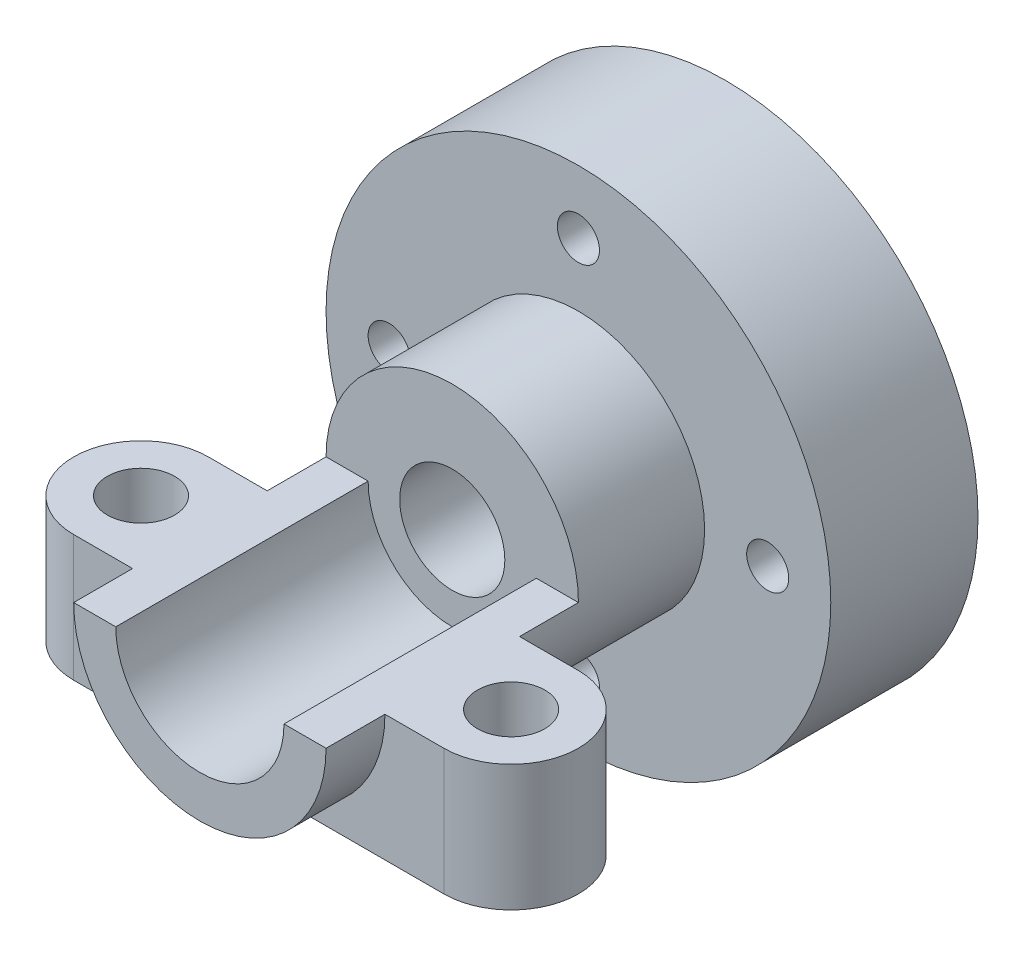
ISO-10303-21;
HEADER;
FILE_DESCRIPTION(('STEP AP214'),'2;1');
FILE_NAME('part.step','',(''),(''),'','','');
FILE_SCHEMA(('AUTOMOTIVE_DESIGN { 1 0 10303 214 1 1 1 1 }'));
ENDSEC;
DATA;
#1=APPLICATION_CONTEXT('core data for automotive mechanical design processes');
#2=APPLICATION_PROTOCOL_DEFINITION('international standard','automotive_design',2000,#1);
#3=PRODUCT_CONTEXT('',#1,'mechanical');
#4=PRODUCT('Part','Part','',(#3));
#5=PRODUCT_RELATED_PRODUCT_CATEGORY('part','',(#4));
#6=PRODUCT_DEFINITION_FORMATION('','',#4);
#7=PRODUCT_DEFINITION_CONTEXT('part definition',#1,'design');
#8=PRODUCT_DEFINITION('design','',#6,#7);
#9=PRODUCT_DEFINITION_SHAPE('','',#8);
#10=(LENGTH_UNIT() NAMED_UNIT(*) SI_UNIT(.MILLI.,.METRE.));
#11=(NAMED_UNIT(*) PLANE_ANGLE_UNIT() SI_UNIT($,.RADIAN.));
#12=(NAMED_UNIT(*) SI_UNIT($,.STERADIAN.) SOLID_ANGLE_UNIT());
#13=UNCERTAINTY_MEASURE_WITH_UNIT(LENGTH_MEASURE(1.E-05),#10,'distance_accuracy_value','');
#14=(GEOMETRIC_REPRESENTATION_CONTEXT(3) GLOBAL_UNCERTAINTY_ASSIGNED_CONTEXT((#13)) GLOBAL_UNIT_ASSIGNED_CONTEXT((#10,
#11,#12)) REPRESENTATION_CONTEXT('',''));
#15=CARTESIAN_POINT('',(0.,0.,0.));
#16=DIRECTION('',(0.,0.,1.));
#17=DIRECTION('',(1.,0.,0.));
#18=AXIS2_PLACEMENT_3D('',#15,#16,#17);
#19=CARTESIAN_POINT('',(-30.,0.,90.));
#20=DIRECTION('',(0.,-1.,0.));
#21=DIRECTION('',(0.,0.,-1.));
#22=AXIS2_PLACEMENT_3D('',#19,#20,#21);
#23=PLANE('',#22);
#24=CARTESIAN_POINT('',(44.,0.,60.));
#25=DIRECTION('',(0.,1.,0.));
#26=DIRECTION('',(0.,0.,1.));
#27=AXIS2_PLACEMENT_3D('',#24,#25,#26);
#28=CIRCLE('',#27,8.);
#29=CARTESIAN_POINT('',(44.,0.,68.));
#30=VERTEX_POINT('',#29);
#31=EDGE_CURVE('E163',#30,#30,#28,.T.);
#32=ORIENTED_EDGE('',*,*,#31,.F.);
#33=EDGE_LOOP('',(#32));
#34=FACE_BOUND('',#33,.T.);
#35=DIRECTION('',(0.,0.,1.));
#36=VECTOR('',#35,1.);
#37=CARTESIAN_POINT('',(20.,0.,30.));
#38=LINE('',#37,#36);
#39=CARTESIAN_POINT('',(20.,0.,30.));
#40=VERTEX_POINT('',#39);
#41=CARTESIAN_POINT('',(20.,0.,90.));
#42=VERTEX_POINT('',#41);
#43=EDGE_CURVE('E198',#40,#42,#38,.T.);
#44=ORIENTED_EDGE('',*,*,#43,.T.);
#45=DIRECTION('',(-1.,0.,0.));
#46=VECTOR('',#45,1.);
#47=CARTESIAN_POINT('',(-30.,0.,90.));
#48=LINE('',#47,#46);
#49=CARTESIAN_POINT('',(30.,0.,90.));
#50=VERTEX_POINT('',#49);
#51=EDGE_CURVE('E230',#50,#42,#48,.T.);
#52=ORIENTED_EDGE('',*,*,#51,.F.);
#53=DIRECTION('',(0.,0.,-1.));
#54=VECTOR('',#53,1.);
#55=CARTESIAN_POINT('',(30.,0.,90.));
#56=LINE('',#55,#54);
#57=CARTESIAN_POINT('',(30.,0.,76.));
#58=VERTEX_POINT('',#57);
#59=EDGE_CURVE('E238',#50,#58,#56,.T.);
#60=ORIENTED_EDGE('',*,*,#59,.T.);
#61=DIRECTION('',(1.,0.,0.));
#62=VECTOR('',#61,1.);
#63=CARTESIAN_POINT('',(30.,0.,76.));
#64=LINE('',#63,#62);
#65=CARTESIAN_POINT('',(44.,0.,76.));
#66=VERTEX_POINT('',#65);
#67=EDGE_CURVE('E151',#58,#66,#64,.T.);
#68=ORIENTED_EDGE('',*,*,#67,.T.);
#69=CARTESIAN_POINT('',(44.,0.,60.));
#70=DIRECTION('',(0.,1.,0.));
#71=DIRECTION('',(0.,0.,1.));
#72=AXIS2_PLACEMENT_3D('',#69,#70,#71);
#73=CIRCLE('',#72,16.);
#74=CARTESIAN_POINT('',(44.,0.,44.));
#75=VERTEX_POINT('',#74);
#76=EDGE_CURVE('E161',#66,#75,#73,.T.);
#77=ORIENTED_EDGE('',*,*,#76,.T.);
#78=DIRECTION('',(-1.,0.,0.));
#79=VECTOR('',#78,1.);
#80=CARTESIAN_POINT('',(44.,0.,44.));
#81=LINE('',#80,#79);
#82=CARTESIAN_POINT('',(30.,0.,44.));
#83=VERTEX_POINT('',#82);
#84=EDGE_CURVE('E146',#75,#83,#81,.T.);
#85=ORIENTED_EDGE('',*,*,#84,.T.);
#86=CARTESIAN_POINT('',(30.,0.,30.));
#87=VERTEX_POINT('',#86);
#88=EDGE_CURVE('E240',#83,#87,#56,.T.);
#89=ORIENTED_EDGE('',*,*,#88,.T.);
#90=DIRECTION('',(-1.,0.,0.));
#91=VECTOR('',#90,1.);
#92=CARTESIAN_POINT('',(-30.,0.,30.));
#93=LINE('',#92,#91);
#94=EDGE_CURVE('E226',#87,#40,#93,.T.);
#95=ORIENTED_EDGE('',*,*,#94,.T.);
#96=EDGE_LOOP('',(#44,#52,#60,#68,#77,#85,#89,#95));
#97=FACE_BOUND('',#96,.T.);
#98=ADVANCED_FACE('F44',(#34,#97),#23,.F.);
#99=CARTESIAN_POINT('',(0.,0.,30.));
#100=DIRECTION('',(0.,0.,-1.));
#101=DIRECTION('',(-1.,0.,0.));
#102=AXIS2_PLACEMENT_3D('',#99,#100,#101);
#103=CYLINDRICAL_SURFACE('',#102,30.);
#104=DIRECTION('',(0.,0.,-1.));
#105=VECTOR('',#104,1.);
#106=CARTESIAN_POINT('',(-30.,0.,90.));
#107=LINE('',#106,#105);
#108=CARTESIAN_POINT('',(-30.,0.,90.));
#109=VERTEX_POINT('',#108);
#110=CARTESIAN_POINT('',(-30.,0.,76.));
#111=VERTEX_POINT('',#110);
#112=EDGE_CURVE('E232',#109,#111,#107,.T.);
#113=ORIENTED_EDGE('',*,*,#112,.T.);
#114=CARTESIAN_POINT('',(0.,0.,76.));
#115=DIRECTION('',(0.,0.,1.));
#116=DIRECTION('',(1.,0.,0.));
#117=AXIS2_PLACEMENT_3D('',#114,#115,#116);
#118=CIRCLE('',#117,30.);
#119=CARTESIAN_POINT('',(0.,-30.,76.));
#120=VERTEX_POINT('',#119);
#121=EDGE_CURVE('E66',#111,#120,#118,.T.);
#122=ORIENTED_EDGE('',*,*,#121,.T.);
#123=EDGE_CURVE('E184',#120,#58,#118,.T.);
#124=ORIENTED_EDGE('',*,*,#123,.T.);
#125=ORIENTED_EDGE('',*,*,#59,.F.);
#126=CARTESIAN_POINT('',(0.,0.,90.));
#127=DIRECTION('',(0.,0.,1.));
#128=DIRECTION('',(1.,0.,0.));
#129=AXIS2_PLACEMENT_3D('',#126,#127,#128);
#130=CIRCLE('',#129,30.);
#131=EDGE_CURVE('E221',#109,#50,#130,.T.);
#132=ORIENTED_EDGE('',*,*,#131,.F.);
#133=EDGE_LOOP('',(#113,#122,#124,#125,#132));
#134=FACE_BOUND('',#133,.T.);
#135=ADVANCED_FACE('F273',(#134),#103,.T.);
#136=CARTESIAN_POINT('',(0.,0.,-35.));
#137=DIRECTION('',(0.,0.,1.));
#138=DIRECTION('',(1.,0.,0.));
#139=AXIS2_PLACEMENT_3D('',#136,#137,#138);
#140=CYLINDRICAL_SURFACE('',#139,60.);
#141=CARTESIAN_POINT('',(0.,0.,-35.));
#142=DIRECTION('',(0.,0.,1.));
#143=DIRECTION('',(1.,0.,0.));
#144=AXIS2_PLACEMENT_3D('',#141,#142,#143);
#145=CIRCLE('',#144,60.);
#146=CARTESIAN_POINT('',(60.,0.,-35.));
#147=VERTEX_POINT('',#146);
#148=EDGE_CURVE('E53',#147,#147,#145,.T.);
#149=ORIENTED_EDGE('',*,*,#148,.T.);
#150=EDGE_LOOP('',(#149));
#151=FACE_BOUND('',#150,.T.);
#152=CARTESIAN_POINT('',(0.,0.,0.));
#153=DIRECTION('',(0.,0.,1.));
#154=DIRECTION('',(1.,0.,0.));
#155=AXIS2_PLACEMENT_3D('',#152,#153,#154);
#156=CIRCLE('',#155,60.);
#157=CARTESIAN_POINT('',(60.,0.,0.));
#158=VERTEX_POINT('',#157);
#159=EDGE_CURVE('E245',#158,#158,#156,.T.);
#160=ORIENTED_EDGE('',*,*,#159,.F.);
#161=EDGE_LOOP('',(#160));
#162=FACE_BOUND('',#161,.T.);
#163=ADVANCED_FACE('F50',(#151,#162),#140,.T.);
#164=CARTESIAN_POINT('',(0.,0.,-35.));
#165=DIRECTION('',(0.,0.,1.));
#166=DIRECTION('',(1.,0.,0.));
#167=AXIS2_PLACEMENT_3D('',#164,#165,#166);
#168=PLANE('',#167);
#169=CARTESIAN_POINT('',(0.,0.,-35.));
#170=DIRECTION('',(0.,0.,-1.));
#171=DIRECTION('',(-1.,0.,0.));
#172=AXIS2_PLACEMENT_3D('',#169,#170,#171);
#173=CIRCLE('',#172,55.);
#174=CARTESIAN_POINT('',(-55.,0.,-35.));
#175=VERTEX_POINT('',#174);
#176=EDGE_CURVE('E216',#175,#175,#173,.T.);
#177=ORIENTED_EDGE('',*,*,#176,.F.);
#178=EDGE_LOOP('',(#177));
#179=FACE_BOUND('',#178,.T.);
#180=ORIENTED_EDGE('',*,*,#148,.F.);
#181=EDGE_LOOP('',(#180));
#182=FACE_BOUND('',#181,.T.);
#183=ADVANCED_FACE('F329',(#179,#182),#168,.F.);
#184=CARTESIAN_POINT('',(0.,0.,0.));
#185=DIRECTION('',(0.,0.,1.));
#186=DIRECTION('',(1.,0.,0.));
#187=AXIS2_PLACEMENT_3D('',#184,#185,#186);
#188=PLANE('',#187);
#189=CARTESIAN_POINT('',(45.,0.,0.));
#190=DIRECTION('',(0.,0.,1.));
#191=DIRECTION('',(1.,0.,0.));
#192=AXIS2_PLACEMENT_3D('',#189,#190,#191);
#193=CIRCLE('',#192,5.);
#194=CARTESIAN_POINT('',(50.,0.,0.));
#195=VERTEX_POINT('',#194);
#196=EDGE_CURVE('E201',#195,#195,#193,.T.);
#197=ORIENTED_EDGE('',*,*,#196,.F.);
#198=EDGE_LOOP('',(#197));
#199=FACE_BOUND('',#198,.T.);
#200=CARTESIAN_POINT('',(0.,45.,0.));
#201=DIRECTION('',(0.,0.,1.));
#202=DIRECTION('',(1.,0.,0.));
#203=AXIS2_PLACEMENT_3D('',#200,#201,#202);
#204=CIRCLE('',#203,5.);
#205=CARTESIAN_POINT('',(5.,45.,0.));
#206=VERTEX_POINT('',#205);
#207=EDGE_CURVE('E206',#206,#206,#204,.T.);
#208=ORIENTED_EDGE('',*,*,#207,.F.);
#209=EDGE_LOOP('',(#208));
#210=FACE_BOUND('',#209,.T.);
#211=CARTESIAN_POINT('',(-45.,0.,0.));
#212=DIRECTION('',(0.,0.,1.));
#213=DIRECTION('',(1.,0.,0.));
#214=AXIS2_PLACEMENT_3D('',#211,#212,#213);
#215=CIRCLE('',#214,5.);
#216=CARTESIAN_POINT('',(-40.,0.,0.));
#217=VERTEX_POINT('',#216);
#218=EDGE_CURVE('E214',#217,#217,#215,.T.);
#219=ORIENTED_EDGE('',*,*,#218,.F.);
#220=EDGE_LOOP('',(#219));
#221=FACE_BOUND('',#220,.T.);
#222=CARTESIAN_POINT('',(0.,-45.,0.));
#223=DIRECTION('',(0.,0.,1.));
#224=DIRECTION('',(1.,0.,0.));
#225=AXIS2_PLACEMENT_3D('',#222,#223,#224);
#226=CIRCLE('',#225,5.);
#227=CARTESIAN_POINT('',(5.,-45.,0.));
#228=VERTEX_POINT('',#227);
#229=EDGE_CURVE('E205',#228,#228,#226,.T.);
#230=ORIENTED_EDGE('',*,*,#229,.F.);
#231=EDGE_LOOP('',(#230));
#232=FACE_BOUND('',#231,.T.);
#233=CARTESIAN_POINT('',(0.,0.,0.));
#234=DIRECTION('',(0.,0.,1.));
#235=DIRECTION('',(1.,0.,0.));
#236=AXIS2_PLACEMENT_3D('',#233,#234,#235);
#237=CIRCLE('',#236,30.);
#238=CARTESIAN_POINT('',(30.,0.,0.));
#239=VERTEX_POINT('',#238);
#240=EDGE_CURVE('E11',#239,#239,#237,.T.);
#241=ORIENTED_EDGE('',*,*,#240,.F.);
#242=EDGE_LOOP('',(#241));
#243=FACE_BOUND('',#242,.T.);
#244=ORIENTED_EDGE('',*,*,#159,.T.);
#245=EDGE_LOOP('',(#244));
#246=FACE_BOUND('',#245,.T.);
#247=ADVANCED_FACE('F321',(#199,#210,#221,#232,#243,#246),#188,.T.);
#248=ORIENTED_EDGE('',*,*,#88,.F.);
#249=CARTESIAN_POINT('',(0.,0.,44.));
#250=DIRECTION('',(0.,0.,-1.));
#251=DIRECTION('',(-1.,0.,0.));
#252=AXIS2_PLACEMENT_3D('',#249,#250,#251);
#253=CIRCLE('',#252,30.);
#254=CARTESIAN_POINT('',(0.,-30.,44.));
#255=VERTEX_POINT('',#254);
#256=EDGE_CURVE('E61',#83,#255,#253,.T.);
#257=ORIENTED_EDGE('',*,*,#256,.T.);
#258=CARTESIAN_POINT('',(-30.,0.,44.));
#259=VERTEX_POINT('',#258);
#260=EDGE_CURVE('E190',#255,#259,#253,.T.);
#261=ORIENTED_EDGE('',*,*,#260,.T.);
#262=CARTESIAN_POINT('',(-30.,0.,30.));
#263=VERTEX_POINT('',#262);
#264=EDGE_CURVE('E235',#259,#263,#107,.T.);
#265=ORIENTED_EDGE('',*,*,#264,.T.);
#266=CARTESIAN_POINT('',(0.,0.,30.));
#267=DIRECTION('',(0.,0.,1.));
#268=DIRECTION('',(1.,0.,0.));
#269=AXIS2_PLACEMENT_3D('',#266,#267,#268);
#270=CIRCLE('',#269,30.);
#271=EDGE_CURVE('E239',#87,#263,#270,.T.);
#272=ORIENTED_EDGE('',*,*,#271,.F.);
#273=EDGE_LOOP('',(#248,#257,#261,#265,#272));
#274=FACE_BOUND('',#273,.T.);
#275=ORIENTED_EDGE('',*,*,#240,.T.);
#276=EDGE_LOOP('',(#275));
#277=FACE_BOUND('',#276,.T.);
#278=ADVANCED_FACE('F304',(#274,#277),#103,.T.);
#279=CARTESIAN_POINT('',(0.,0.,30.));
#280=DIRECTION('',(0.,0.,1.));
#281=DIRECTION('',(1.,0.,0.));
#282=AXIS2_PLACEMENT_3D('',#279,#280,#281);
#283=PLANE('',#282);
#284=CARTESIAN_POINT('',(0.,0.,30.));
#285=DIRECTION('',(0.,0.,1.));
#286=DIRECTION('',(1.,0.,0.));
#287=AXIS2_PLACEMENT_3D('',#284,#285,#286);
#288=CIRCLE('',#287,12.5);
#289=CARTESIAN_POINT('',(12.5,0.,30.));
#290=VERTEX_POINT('',#289);
#291=EDGE_CURVE('E186',#290,#290,#288,.T.);
#292=ORIENTED_EDGE('',*,*,#291,.F.);
#293=EDGE_LOOP('',(#292));
#294=FACE_BOUND('',#293,.T.);
#295=ORIENTED_EDGE('',*,*,#94,.F.);
#296=ORIENTED_EDGE('',*,*,#271,.T.);
#297=CARTESIAN_POINT('',(-20.,0.,30.));
#298=VERTEX_POINT('',#297);
#299=EDGE_CURVE('E220',#298,#263,#93,.T.);
#300=ORIENTED_EDGE('',*,*,#299,.F.);
#301=CARTESIAN_POINT('',(0.,0.,30.));
#302=DIRECTION('',(0.,0.,1.));
#303=DIRECTION('',(1.,0.,0.));
#304=AXIS2_PLACEMENT_3D('',#301,#302,#303);
#305=CIRCLE('',#304,20.);
#306=EDGE_CURVE('E195',#298,#40,#305,.T.);
#307=ORIENTED_EDGE('',*,*,#306,.T.);
#308=EDGE_LOOP('',(#295,#296,#300,#307));
#309=FACE_BOUND('',#308,.T.);
#310=ADVANCED_FACE('F315',(#294,#309),#283,.T.);
#311=CARTESIAN_POINT('',(-44.,0.,60.));
#312=DIRECTION('',(0.,1.,0.));
#313=DIRECTION('',(0.,0.,1.));
#314=AXIS2_PLACEMENT_3D('',#311,#312,#313);
#315=CIRCLE('',#314,8.00000000000001);
#316=CARTESIAN_POINT('',(-44.,0.,68.));
#317=VERTEX_POINT('',#316);
#318=EDGE_CURVE('E263',#317,#317,#315,.T.);
#319=ORIENTED_EDGE('',*,*,#318,.F.);
#320=EDGE_LOOP('',(#319));
#321=FACE_BOUND('',#320,.T.);
#322=CARTESIAN_POINT('',(-20.,0.,90.));
#323=VERTEX_POINT('',#322);
#324=EDGE_CURVE('E227',#323,#109,#48,.T.);
#325=ORIENTED_EDGE('',*,*,#324,.F.);
#326=DIRECTION('',(0.,0.,1.));
#327=VECTOR('',#326,1.);
#328=CARTESIAN_POINT('',(-20.,0.,30.));
#329=LINE('',#328,#327);
#330=EDGE_CURVE('E196',#298,#323,#329,.T.);
#331=ORIENTED_EDGE('',*,*,#330,.F.);
#332=ORIENTED_EDGE('',*,*,#299,.T.);
#333=ORIENTED_EDGE('',*,*,#264,.F.);
#334=DIRECTION('',(-1.,0.,0.));
#335=VECTOR('',#334,1.);
#336=CARTESIAN_POINT('',(-30.,0.,44.));
#337=LINE('',#336,#335);
#338=CARTESIAN_POINT('',(-44.,0.,44.));
#339=VERTEX_POINT('',#338);
#340=EDGE_CURVE('E175',#259,#339,#337,.T.);
#341=ORIENTED_EDGE('',*,*,#340,.T.);
#342=CARTESIAN_POINT('',(-44.,0.,60.));
#343=DIRECTION('',(0.,1.,0.));
#344=DIRECTION('',(0.,0.,1.));
#345=AXIS2_PLACEMENT_3D('',#342,#343,#344);
#346=CIRCLE('',#345,16.);
#347=CARTESIAN_POINT('',(-44.,0.,76.));
#348=VERTEX_POINT('',#347);
#349=EDGE_CURVE('E168',#339,#348,#346,.T.);
#350=ORIENTED_EDGE('',*,*,#349,.T.);
#351=DIRECTION('',(1.,0.,0.));
#352=VECTOR('',#351,1.);
#353=CARTESIAN_POINT('',(-44.,0.,76.));
#354=LINE('',#353,#352);
#355=EDGE_CURVE('E174',#348,#111,#354,.T.);
#356=ORIENTED_EDGE('',*,*,#355,.T.);
#357=ORIENTED_EDGE('',*,*,#112,.F.);
#358=EDGE_LOOP('',(#325,#331,#332,#333,#341,#350,#356,#357));
#359=FACE_BOUND('',#358,.T.);
#360=ADVANCED_FACE('F276',(#321,#359),#23,.F.);
#361=CARTESIAN_POINT('',(0.,0.,90.));
#362=DIRECTION('',(0.,0.,1.));
#363=DIRECTION('',(1.,0.,0.));
#364=AXIS2_PLACEMENT_3D('',#361,#362,#363);
#365=PLANE('',#364);
#366=CARTESIAN_POINT('',(0.,0.,90.));
#367=DIRECTION('',(0.,0.,1.));
#368=DIRECTION('',(1.,0.,0.));
#369=AXIS2_PLACEMENT_3D('',#366,#367,#368);
#370=CIRCLE('',#369,20.);
#371=EDGE_CURVE('E199',#323,#42,#370,.T.);
#372=ORIENTED_EDGE('',*,*,#371,.F.);
#373=ORIENTED_EDGE('',*,*,#324,.T.);
#374=ORIENTED_EDGE('',*,*,#131,.T.);
#375=ORIENTED_EDGE('',*,*,#51,.T.);
#376=EDGE_LOOP('',(#372,#373,#374,#375));
#377=FACE_BOUND('',#376,.T.);
#378=ADVANCED_FACE('F281',(#377),#365,.T.);
#379=CARTESIAN_POINT('',(0.,0.,-20.));
#380=DIRECTION('',(0.,0.,-1.));
#381=DIRECTION('',(-1.,0.,0.));
#382=AXIS2_PLACEMENT_3D('',#379,#380,#381);
#383=CYLINDRICAL_SURFACE('',#382,55.);
#384=CARTESIAN_POINT('',(0.,0.,-20.));
#385=DIRECTION('',(0.,0.,-1.));
#386=DIRECTION('',(-1.,0.,0.));
#387=AXIS2_PLACEMENT_3D('',#384,#385,#386);
#388=CIRCLE('',#387,55.);
#389=CARTESIAN_POINT('',(-55.,0.,-20.));
#390=VERTEX_POINT('',#389);
#391=EDGE_CURVE('E218',#390,#390,#388,.T.);
#392=ORIENTED_EDGE('',*,*,#391,.F.);
#393=EDGE_LOOP('',(#392));
#394=FACE_BOUND('',#393,.T.);
#395=ORIENTED_EDGE('',*,*,#176,.T.);
#396=EDGE_LOOP('',(#395));
#397=FACE_BOUND('',#396,.T.);
#398=ADVANCED_FACE('F515',(#394,#397),#383,.F.);
#399=CARTESIAN_POINT('',(0.,0.,-20.));
#400=DIRECTION('',(0.,0.,-1.));
#401=DIRECTION('',(-1.,0.,0.));
#402=AXIS2_PLACEMENT_3D('',#399,#400,#401);
#403=PLANE('',#402);
#404=CARTESIAN_POINT('',(0.,0.,-20.));
#405=DIRECTION('',(0.,0.,-1.));
#406=DIRECTION('',(-1.,0.,0.));
#407=AXIS2_PLACEMENT_3D('',#404,#405,#406);
#408=CIRCLE('',#407,12.5);
#409=CARTESIAN_POINT('',(-12.5,0.,-20.));
#410=VERTEX_POINT('',#409);
#411=EDGE_CURVE('E191',#410,#410,#408,.T.);
#412=ORIENTED_EDGE('',*,*,#411,.F.);
#413=EDGE_LOOP('',(#412));
#414=FACE_BOUND('',#413,.T.);
#415=CARTESIAN_POINT('',(45.,0.,-20.));
#416=DIRECTION('',(0.,0.,-1.));
#417=DIRECTION('',(-1.,0.,0.));
#418=AXIS2_PLACEMENT_3D('',#415,#416,#417);
#419=CIRCLE('',#418,5.);
#420=CARTESIAN_POINT('',(50.,0.,-20.));
#421=VERTEX_POINT('',#420);
#422=EDGE_CURVE('E224',#421,#421,#419,.T.);
#423=ORIENTED_EDGE('',*,*,#422,.F.);
#424=EDGE_LOOP('',(#423));
#425=FACE_BOUND('',#424,.T.);
#426=CARTESIAN_POINT('',(0.,45.,-20.));
#427=DIRECTION('',(0.,0.,-1.));
#428=DIRECTION('',(-1.,0.,0.));
#429=AXIS2_PLACEMENT_3D('',#426,#427,#428);
#430=CIRCLE('',#429,5.);
#431=CARTESIAN_POINT('',(5.,45.,-20.));
#432=VERTEX_POINT('',#431);
#433=EDGE_CURVE('E254',#432,#432,#430,.T.);
#434=ORIENTED_EDGE('',*,*,#433,.F.);
#435=EDGE_LOOP('',(#434));
#436=FACE_BOUND('',#435,.T.);
#437=CARTESIAN_POINT('',(-45.,0.,-20.));
#438=DIRECTION('',(0.,0.,-1.));
#439=DIRECTION('',(-1.,0.,0.));
#440=AXIS2_PLACEMENT_3D('',#437,#438,#439);
#441=CIRCLE('',#440,5.);
#442=CARTESIAN_POINT('',(-40.,0.,-20.));
#443=VERTEX_POINT('',#442);
#444=EDGE_CURVE('E249',#443,#443,#441,.T.);
#445=ORIENTED_EDGE('',*,*,#444,.F.);
#446=EDGE_LOOP('',(#445));
#447=FACE_BOUND('',#446,.T.);
#448=CARTESIAN_POINT('',(0.,-45.,-20.));
#449=DIRECTION('',(0.,0.,-1.));
#450=DIRECTION('',(-1.,0.,0.));
#451=AXIS2_PLACEMENT_3D('',#448,#449,#450);
#452=CIRCLE('',#451,5.);
#453=CARTESIAN_POINT('',(5.,-45.,-20.));
#454=VERTEX_POINT('',#453);
#455=EDGE_CURVE('E210',#454,#454,#452,.T.);
#456=ORIENTED_EDGE('',*,*,#455,.F.);
#457=EDGE_LOOP('',(#456));
#458=FACE_BOUND('',#457,.T.);
#459=ORIENTED_EDGE('',*,*,#391,.T.);
#460=EDGE_LOOP('',(#459));
#461=FACE_BOUND('',#460,.T.);
#462=ADVANCED_FACE('F504',(#414,#425,#436,#447,#458,#461),#403,.T.);
#463=CARTESIAN_POINT('',(0.,-45.,-52.));
#464=DIRECTION('',(0.,0.,1.));
#465=DIRECTION('',(1.,0.,0.));
#466=AXIS2_PLACEMENT_3D('',#463,#464,#465);
#467=CYLINDRICAL_SURFACE('',#466,5.);
#468=CARTESIAN_POINT('',(5.,-45.,-20.));
#469=CARTESIAN_POINT('',(5.,-45.,-19.7916666666667));
#470=CARTESIAN_POINT('',(5.,-45.,-19.5833333333333));
#471=CARTESIAN_POINT('',(5.,-45.,-19.1666666666667));
#472=CARTESIAN_POINT('',(5.,-45.,-18.9583333333333));
#473=CARTESIAN_POINT('',(5.,-45.,-18.5416666666667));
#474=CARTESIAN_POINT('',(5.,-45.,-18.3333333333333));
#475=CARTESIAN_POINT('',(5.,-45.,-17.9166666666667));
#476=CARTESIAN_POINT('',(5.,-45.,-17.7083333333333));
#477=CARTESIAN_POINT('',(5.,-45.,-17.2916666666667));
#478=CARTESIAN_POINT('',(5.,-45.,-17.0833333333333));
#479=CARTESIAN_POINT('',(5.,-45.,-16.6666666666667));
#480=CARTESIAN_POINT('',(5.,-45.,-16.4583333333333));
#481=CARTESIAN_POINT('',(5.,-45.,-16.0416666666667));
#482=CARTESIAN_POINT('',(5.,-45.,-15.8333333333333));
#483=CARTESIAN_POINT('',(5.,-45.,-15.4166666666667));
#484=CARTESIAN_POINT('',(5.,-45.,-15.2083333333333));
#485=CARTESIAN_POINT('',(5.,-45.,-14.7916666666667));
#486=CARTESIAN_POINT('',(5.,-45.,-14.5833333333333));
#487=CARTESIAN_POINT('',(5.,-45.,-14.1666666666667));
#488=CARTESIAN_POINT('',(5.,-45.,-13.9583333333333));
#489=CARTESIAN_POINT('',(5.,-45.,-13.5416666666667));
#490=CARTESIAN_POINT('',(5.,-45.,-13.3333333333333));
#491=CARTESIAN_POINT('',(5.,-45.,-12.9166666666667));
#492=CARTESIAN_POINT('',(5.,-45.,-12.7083333333333));
#493=CARTESIAN_POINT('',(5.,-45.,-12.2916666666667));
#494=CARTESIAN_POINT('',(5.,-45.,-12.0833333333333));
#495=CARTESIAN_POINT('',(5.,-45.,-11.6666666666667));
#496=CARTESIAN_POINT('',(5.,-45.,-11.4583333333333));
#497=CARTESIAN_POINT('',(5.,-45.,-11.0416666666667));
#498=CARTESIAN_POINT('',(5.,-45.,-10.8333333333333));
#499=CARTESIAN_POINT('',(5.,-45.,-10.4166666666667));
#500=CARTESIAN_POINT('',(5.,-45.,-10.2083333333333));
#501=CARTESIAN_POINT('',(5.,-45.,-9.79166666666667));
#502=CARTESIAN_POINT('',(5.,-45.,-9.58333333333333));
#503=CARTESIAN_POINT('',(5.,-45.,-9.16666666666667));
#504=CARTESIAN_POINT('',(5.,-45.,-8.95833333333333));
#505=CARTESIAN_POINT('',(5.,-45.,-8.54166666666667));
#506=CARTESIAN_POINT('',(5.,-45.,-8.33333333333333));
#507=CARTESIAN_POINT('',(5.,-45.,-7.91666666666667));
#508=CARTESIAN_POINT('',(5.,-45.,-7.70833333333333));
#509=CARTESIAN_POINT('',(5.,-45.,-7.29166666666667));
#510=CARTESIAN_POINT('',(5.,-45.,-7.08333333333333));
#511=CARTESIAN_POINT('',(5.,-45.,-6.66666666666667));
#512=CARTESIAN_POINT('',(5.,-45.,-6.45833333333334));
#513=CARTESIAN_POINT('',(5.,-45.,-6.04166666666667));
#514=CARTESIAN_POINT('',(5.,-45.,-5.83333333333334));
#515=CARTESIAN_POINT('',(5.,-45.,-5.41666666666667));
#516=CARTESIAN_POINT('',(5.,-45.,-5.20833333333334));
#517=CARTESIAN_POINT('',(5.,-45.,-4.79166666666667));
#518=CARTESIAN_POINT('',(5.,-45.,-4.58333333333334));
#519=CARTESIAN_POINT('',(5.,-45.,-4.16666666666667));
#520=CARTESIAN_POINT('',(5.,-45.,-3.95833333333334));
#521=CARTESIAN_POINT('',(5.,-45.,-3.54166666666667));
#522=CARTESIAN_POINT('',(5.,-45.,-3.33333333333334));
#523=CARTESIAN_POINT('',(5.,-45.,-2.91666666666667));
#524=CARTESIAN_POINT('',(5.,-45.,-2.70833333333334));
#525=CARTESIAN_POINT('',(5.,-45.,-2.29166666666667));
#526=CARTESIAN_POINT('',(5.,-45.,-2.08333333333334));
#527=CARTESIAN_POINT('',(5.,-45.,-1.66666666666667));
#528=CARTESIAN_POINT('',(5.,-45.,-1.45833333333333));
#529=CARTESIAN_POINT('',(5.,-45.,-1.04166666666667));
#530=CARTESIAN_POINT('',(5.,-45.,-0.833333333333334));
#531=CARTESIAN_POINT('',(5.,-45.,-0.416666666666667));
#532=CARTESIAN_POINT('',(5.,-45.,-0.208333333333334));
#533=CARTESIAN_POINT('',(5.,-45.,0.));
#534=B_SPLINE_CURVE_WITH_KNOTS('',3,(#468,#469,#470,#471,#472,#473,#474,#475,#476,#477,#478,
#479,#480,#481,#482,#483,#484,#485,#486,#487,#488,#489,#490,#491,#492,#493,#494,#495,#496,#497,
#498,#499,#500,#501,#502,#503,#504,#505,#506,#507,#508,#509,#510,#511,#512,#513,#514,#515,#516,
#517,#518,#519,#520,#521,#522,#523,#524,#525,#526,#527,#528,#529,#530,#531,#532,#533),
.UNSPECIFIED.,.F.,.F.,(4,2,2,2,2,2,2,2,2,2,2,2,2,2,2,2,2,2,2,2,2,2,2,2,2,2,2,2,2,2,2,2,4),(0.,
0.625000000000001,1.25,1.875,2.5,3.125,3.75,4.375,5.,5.62500000000001,6.25,6.875,7.5,8.125,8.75,
9.375,10.,10.625,11.25,11.875,12.5,13.125,13.75,14.375,15.,15.625,16.25,16.875,17.5,18.125,
18.75,19.375,20.),.UNSPECIFIED.);
#535=EDGE_CURVE('BSEAM500',#454,#228,#534,.T.);
#536=ORIENTED_EDGE('',*,*,#455,.T.);
#537=ORIENTED_EDGE('',*,*,#229,.T.);
#538=ORIENTED_EDGE('',*,*,#535,.T.);
#539=ORIENTED_EDGE('',*,*,#535,.F.);
#540=EDGE_LOOP('',(#536,#538,#537,#539));
#541=FACE_BOUND('',#540,.T.);
#542=ADVANCED_FACE('F500',(#541),#467,.F.);
#543=CARTESIAN_POINT('',(-45.,0.,-52.));
#544=DIRECTION('',(0.,0.,1.));
#545=DIRECTION('',(1.,0.,0.));
#546=AXIS2_PLACEMENT_3D('',#543,#544,#545);
#547=CYLINDRICAL_SURFACE('',#546,5.);
#548=CARTESIAN_POINT('',(-40.,0.,-20.));
#549=CARTESIAN_POINT('',(-40.,0.,-19.7916666666667));
#550=CARTESIAN_POINT('',(-40.,0.,-19.5833333333333));
#551=CARTESIAN_POINT('',(-40.,0.,-19.1666666666667));
#552=CARTESIAN_POINT('',(-40.,0.,-18.9583333333333));
#553=CARTESIAN_POINT('',(-40.,0.,-18.5416666666667));
#554=CARTESIAN_POINT('',(-40.,0.,-18.3333333333333));
#555=CARTESIAN_POINT('',(-40.,0.,-17.9166666666667));
#556=CARTESIAN_POINT('',(-40.,0.,-17.7083333333333));
#557=CARTESIAN_POINT('',(-40.,0.,-17.2916666666667));
#558=CARTESIAN_POINT('',(-40.,0.,-17.0833333333333));
#559=CARTESIAN_POINT('',(-40.,0.,-16.6666666666667));
#560=CARTESIAN_POINT('',(-40.,0.,-16.4583333333333));
#561=CARTESIAN_POINT('',(-40.,0.,-16.0416666666667));
#562=CARTESIAN_POINT('',(-40.,0.,-15.8333333333333));
#563=CARTESIAN_POINT('',(-40.,0.,-15.4166666666667));
#564=CARTESIAN_POINT('',(-40.,0.,-15.2083333333333));
#565=CARTESIAN_POINT('',(-40.,0.,-14.7916666666667));
#566=CARTESIAN_POINT('',(-40.,0.,-14.5833333333333));
#567=CARTESIAN_POINT('',(-40.,0.,-14.1666666666667));
#568=CARTESIAN_POINT('',(-40.,0.,-13.9583333333333));
#569=CARTESIAN_POINT('',(-40.,0.,-13.5416666666667));
#570=CARTESIAN_POINT('',(-40.,0.,-13.3333333333333));
#571=CARTESIAN_POINT('',(-40.,0.,-12.9166666666667));
#572=CARTESIAN_POINT('',(-40.,0.,-12.7083333333333));
#573=CARTESIAN_POINT('',(-40.,0.,-12.2916666666667));
#574=CARTESIAN_POINT('',(-40.,0.,-12.0833333333333));
#575=CARTESIAN_POINT('',(-40.,0.,-11.6666666666667));
#576=CARTESIAN_POINT('',(-40.,0.,-11.4583333333333));
#577=CARTESIAN_POINT('',(-40.,0.,-11.0416666666667));
#578=CARTESIAN_POINT('',(-40.,0.,-10.8333333333333));
#579=CARTESIAN_POINT('',(-40.,0.,-10.4166666666667));
#580=CARTESIAN_POINT('',(-40.,0.,-10.2083333333333));
#581=CARTESIAN_POINT('',(-40.,0.,-9.79166666666667));
#582=CARTESIAN_POINT('',(-40.,0.,-9.58333333333333));
#583=CARTESIAN_POINT('',(-40.,0.,-9.16666666666667));
#584=CARTESIAN_POINT('',(-40.,0.,-8.95833333333333));
#585=CARTESIAN_POINT('',(-40.,0.,-8.54166666666667));
#586=CARTESIAN_POINT('',(-40.,0.,-8.33333333333333));
#587=CARTESIAN_POINT('',(-40.,0.,-7.91666666666667));
#588=CARTESIAN_POINT('',(-40.,0.,-7.70833333333333));
#589=CARTESIAN_POINT('',(-40.,0.,-7.29166666666667));
#590=CARTESIAN_POINT('',(-40.,0.,-7.08333333333333));
#591=CARTESIAN_POINT('',(-40.,0.,-6.66666666666667));
#592=CARTESIAN_POINT('',(-40.,0.,-6.45833333333334));
#593=CARTESIAN_POINT('',(-40.,0.,-6.04166666666667));
#594=CARTESIAN_POINT('',(-40.,0.,-5.83333333333334));
#595=CARTESIAN_POINT('',(-40.,0.,-5.41666666666667));
#596=CARTESIAN_POINT('',(-40.,0.,-5.20833333333334));
#597=CARTESIAN_POINT('',(-40.,0.,-4.79166666666667));
#598=CARTESIAN_POINT('',(-40.,0.,-4.58333333333334));
#599=CARTESIAN_POINT('',(-40.,0.,-4.16666666666667));
#600=CARTESIAN_POINT('',(-40.,0.,-3.95833333333334));
#601=CARTESIAN_POINT('',(-40.,0.,-3.54166666666667));
#602=CARTESIAN_POINT('',(-40.,0.,-3.33333333333334));
#603=CARTESIAN_POINT('',(-40.,0.,-2.91666666666667));
#604=CARTESIAN_POINT('',(-40.,0.,-2.70833333333334));
#605=CARTESIAN_POINT('',(-40.,0.,-2.29166666666667));
#606=CARTESIAN_POINT('',(-40.,0.,-2.08333333333334));
#607=CARTESIAN_POINT('',(-40.,0.,-1.66666666666667));
#608=CARTESIAN_POINT('',(-40.,0.,-1.45833333333333));
#609=CARTESIAN_POINT('',(-40.,0.,-1.04166666666667));
#610=CARTESIAN_POINT('',(-40.,0.,-0.833333333333334));
#611=CARTESIAN_POINT('',(-40.,0.,-0.416666666666667));
#612=CARTESIAN_POINT('',(-40.,0.,-0.208333333333334));
#613=CARTESIAN_POINT('',(-40.,0.,0.));
#614=B_SPLINE_CURVE_WITH_KNOTS('',3,(#548,#549,#550,#551,#552,#553,#554,#555,#556,#557,#558,
#559,#560,#561,#562,#563,#564,#565,#566,#567,#568,#569,#570,#571,#572,#573,#574,#575,#576,#577,
#578,#579,#580,#581,#582,#583,#584,#585,#586,#587,#588,#589,#590,#591,#592,#593,#594,#595,#596,
#597,#598,#599,#600,#601,#602,#603,#604,#605,#606,#607,#608,#609,#610,#611,#612,#613),
.UNSPECIFIED.,.F.,.F.,(4,2,2,2,2,2,2,2,2,2,2,2,2,2,2,2,2,2,2,2,2,2,2,2,2,2,2,2,2,2,2,2,4),(0.,
0.625000000000001,1.25,1.875,2.5,3.125,3.75,4.375,5.,5.62500000000001,6.25,6.875,7.5,8.125,8.75,
9.375,10.,10.625,11.25,11.875,12.5,13.125,13.75,14.375,15.,15.625,16.25,16.875,17.5,18.125,
18.75,19.375,20.),.UNSPECIFIED.);
#615=EDGE_CURVE('BSEAM490',#443,#217,#614,.T.);
#616=ORIENTED_EDGE('',*,*,#444,.T.);
#617=ORIENTED_EDGE('',*,*,#218,.T.);
#618=ORIENTED_EDGE('',*,*,#615,.T.);
#619=ORIENTED_EDGE('',*,*,#615,.F.);
#620=EDGE_LOOP('',(#616,#618,#617,#619));
#621=FACE_BOUND('',#620,.T.);
#622=ADVANCED_FACE('F490',(#621),#547,.F.);
#623=CARTESIAN_POINT('',(0.,45.,-52.));
#624=DIRECTION('',(0.,0.,1.));
#625=DIRECTION('',(1.,0.,0.));
#626=AXIS2_PLACEMENT_3D('',#623,#624,#625);
#627=CYLINDRICAL_SURFACE('',#626,5.);
#628=CARTESIAN_POINT('',(5.,45.,-20.));
#629=CARTESIAN_POINT('',(5.,45.,-19.7916666666667));
#630=CARTESIAN_POINT('',(5.,45.,-19.5833333333333));
#631=CARTESIAN_POINT('',(5.,45.,-19.1666666666667));
#632=CARTESIAN_POINT('',(5.,45.,-18.9583333333333));
#633=CARTESIAN_POINT('',(5.,45.,-18.5416666666667));
#634=CARTESIAN_POINT('',(5.,45.,-18.3333333333333));
#635=CARTESIAN_POINT('',(5.,45.,-17.9166666666667));
#636=CARTESIAN_POINT('',(5.,45.,-17.7083333333333));
#637=CARTESIAN_POINT('',(5.,45.,-17.2916666666667));
#638=CARTESIAN_POINT('',(5.,45.,-17.0833333333333));
#639=CARTESIAN_POINT('',(5.,45.,-16.6666666666667));
#640=CARTESIAN_POINT('',(5.,45.,-16.4583333333333));
#641=CARTESIAN_POINT('',(5.,45.,-16.0416666666667));
#642=CARTESIAN_POINT('',(5.,45.,-15.8333333333333));
#643=CARTESIAN_POINT('',(5.,45.,-15.4166666666667));
#644=CARTESIAN_POINT('',(5.,45.,-15.2083333333333));
#645=CARTESIAN_POINT('',(5.,45.,-14.7916666666667));
#646=CARTESIAN_POINT('',(5.,45.,-14.5833333333333));
#647=CARTESIAN_POINT('',(5.,45.,-14.1666666666667));
#648=CARTESIAN_POINT('',(5.,45.,-13.9583333333333));
#649=CARTESIAN_POINT('',(5.,45.,-13.5416666666667));
#650=CARTESIAN_POINT('',(5.,45.,-13.3333333333333));
#651=CARTESIAN_POINT('',(5.,45.,-12.9166666666667));
#652=CARTESIAN_POINT('',(5.,45.,-12.7083333333333));
#653=CARTESIAN_POINT('',(5.,45.,-12.2916666666667));
#654=CARTESIAN_POINT('',(5.,45.,-12.0833333333333));
#655=CARTESIAN_POINT('',(5.,45.,-11.6666666666667));
#656=CARTESIAN_POINT('',(5.,45.,-11.4583333333333));
#657=CARTESIAN_POINT('',(5.,45.,-11.0416666666667));
#658=CARTESIAN_POINT('',(5.,45.,-10.8333333333333));
#659=CARTESIAN_POINT('',(5.,45.,-10.4166666666667));
#660=CARTESIAN_POINT('',(5.,45.,-10.2083333333333));
#661=CARTESIAN_POINT('',(5.,45.,-9.79166666666667));
#662=CARTESIAN_POINT('',(5.,45.,-9.58333333333333));
#663=CARTESIAN_POINT('',(5.,45.,-9.16666666666667));
#664=CARTESIAN_POINT('',(5.,45.,-8.95833333333333));
#665=CARTESIAN_POINT('',(5.,45.,-8.54166666666667));
#666=CARTESIAN_POINT('',(5.,45.,-8.33333333333333));
#667=CARTESIAN_POINT('',(5.,45.,-7.91666666666667));
#668=CARTESIAN_POINT('',(5.,45.,-7.70833333333333));
#669=CARTESIAN_POINT('',(5.,45.,-7.29166666666667));
#670=CARTESIAN_POINT('',(5.,45.,-7.08333333333333));
#671=CARTESIAN_POINT('',(5.,45.,-6.66666666666667));
#672=CARTESIAN_POINT('',(5.,45.,-6.45833333333334));
#673=CARTESIAN_POINT('',(5.,45.,-6.04166666666667));
#674=CARTESIAN_POINT('',(5.,45.,-5.83333333333334));
#675=CARTESIAN_POINT('',(5.,45.,-5.41666666666667));
#676=CARTESIAN_POINT('',(5.,45.,-5.20833333333334));
#677=CARTESIAN_POINT('',(5.,45.,-4.79166666666667));
#678=CARTESIAN_POINT('',(5.,45.,-4.58333333333334));
#679=CARTESIAN_POINT('',(5.,45.,-4.16666666666667));
#680=CARTESIAN_POINT('',(5.,45.,-3.95833333333334));
#681=CARTESIAN_POINT('',(5.,45.,-3.54166666666667));
#682=CARTESIAN_POINT('',(5.,45.,-3.33333333333334));
#683=CARTESIAN_POINT('',(5.,45.,-2.91666666666667));
#684=CARTESIAN_POINT('',(5.,45.,-2.70833333333334));
#685=CARTESIAN_POINT('',(5.,45.,-2.29166666666667));
#686=CARTESIAN_POINT('',(5.,45.,-2.08333333333334));
#687=CARTESIAN_POINT('',(5.,45.,-1.66666666666667));
#688=CARTESIAN_POINT('',(5.,45.,-1.45833333333333));
#689=CARTESIAN_POINT('',(5.,45.,-1.04166666666667));
#690=CARTESIAN_POINT('',(5.,45.,-0.833333333333334));
#691=CARTESIAN_POINT('',(5.,45.,-0.416666666666667));
#692=CARTESIAN_POINT('',(5.,45.,-0.208333333333334));
#693=CARTESIAN_POINT('',(5.,45.,0.));
#694=B_SPLINE_CURVE_WITH_KNOTS('',3,(#628,#629,#630,#631,#632,#633,#634,#635,#636,#637,#638,
#639,#640,#641,#642,#643,#644,#645,#646,#647,#648,#649,#650,#651,#652,#653,#654,#655,#656,#657,
#658,#659,#660,#661,#662,#663,#664,#665,#666,#667,#668,#669,#670,#671,#672,#673,#674,#675,#676,
#677,#678,#679,#680,#681,#682,#683,#684,#685,#686,#687,#688,#689,#690,#691,#692,#693),
.UNSPECIFIED.,.F.,.F.,(4,2,2,2,2,2,2,2,2,2,2,2,2,2,2,2,2,2,2,2,2,2,2,2,2,2,2,2,2,2,2,2,4),(0.,
0.625000000000001,1.25,1.875,2.5,3.125,3.75,4.375,5.,5.62500000000001,6.25,6.875,7.5,8.125,8.75,
9.375,10.,10.625,11.25,11.875,12.5,13.125,13.75,14.375,15.,15.625,16.25,16.875,17.5,18.125,
18.75,19.375,20.),.UNSPECIFIED.);
#695=EDGE_CURVE('BSEAM482',#432,#206,#694,.T.);
#696=ORIENTED_EDGE('',*,*,#433,.T.);
#697=ORIENTED_EDGE('',*,*,#207,.T.);
#698=ORIENTED_EDGE('',*,*,#695,.T.);
#699=ORIENTED_EDGE('',*,*,#695,.F.);
#700=EDGE_LOOP('',(#696,#698,#697,#699));
#701=FACE_BOUND('',#700,.T.);
#702=ADVANCED_FACE('F482',(#701),#627,.F.);
#703=CARTESIAN_POINT('',(45.,0.,-52.));
#704=DIRECTION('',(0.,0.,1.));
#705=DIRECTION('',(1.,0.,0.));
#706=AXIS2_PLACEMENT_3D('',#703,#704,#705);
#707=CYLINDRICAL_SURFACE('',#706,5.);
#708=CARTESIAN_POINT('',(50.,0.,-20.));
#709=CARTESIAN_POINT('',(50.,0.,-19.7916666666667));
#710=CARTESIAN_POINT('',(50.,0.,-19.5833333333333));
#711=CARTESIAN_POINT('',(50.,0.,-19.1666666666667));
#712=CARTESIAN_POINT('',(50.,0.,-18.9583333333333));
#713=CARTESIAN_POINT('',(50.,0.,-18.5416666666667));
#714=CARTESIAN_POINT('',(50.,0.,-18.3333333333333));
#715=CARTESIAN_POINT('',(50.,0.,-17.9166666666667));
#716=CARTESIAN_POINT('',(50.,0.,-17.7083333333333));
#717=CARTESIAN_POINT('',(50.,0.,-17.2916666666667));
#718=CARTESIAN_POINT('',(50.,0.,-17.0833333333333));
#719=CARTESIAN_POINT('',(50.,0.,-16.6666666666667));
#720=CARTESIAN_POINT('',(50.,0.,-16.4583333333333));
#721=CARTESIAN_POINT('',(50.,0.,-16.0416666666667));
#722=CARTESIAN_POINT('',(50.,0.,-15.8333333333333));
#723=CARTESIAN_POINT('',(50.,0.,-15.4166666666667));
#724=CARTESIAN_POINT('',(50.,0.,-15.2083333333333));
#725=CARTESIAN_POINT('',(50.,0.,-14.7916666666667));
#726=CARTESIAN_POINT('',(50.,0.,-14.5833333333333));
#727=CARTESIAN_POINT('',(50.,0.,-14.1666666666667));
#728=CARTESIAN_POINT('',(50.,0.,-13.9583333333333));
#729=CARTESIAN_POINT('',(50.,0.,-13.5416666666667));
#730=CARTESIAN_POINT('',(50.,0.,-13.3333333333333));
#731=CARTESIAN_POINT('',(50.,0.,-12.9166666666667));
#732=CARTESIAN_POINT('',(50.,0.,-12.7083333333333));
#733=CARTESIAN_POINT('',(50.,0.,-12.2916666666667));
#734=CARTESIAN_POINT('',(50.,0.,-12.0833333333333));
#735=CARTESIAN_POINT('',(50.,0.,-11.6666666666667));
#736=CARTESIAN_POINT('',(50.,0.,-11.4583333333333));
#737=CARTESIAN_POINT('',(50.,0.,-11.0416666666667));
#738=CARTESIAN_POINT('',(50.,0.,-10.8333333333333));
#739=CARTESIAN_POINT('',(50.,0.,-10.4166666666667));
#740=CARTESIAN_POINT('',(50.,0.,-10.2083333333333));
#741=CARTESIAN_POINT('',(50.,0.,-9.79166666666667));
#742=CARTESIAN_POINT('',(50.,0.,-9.58333333333333));
#743=CARTESIAN_POINT('',(50.,0.,-9.16666666666667));
#744=CARTESIAN_POINT('',(50.,0.,-8.95833333333333));
#745=CARTESIAN_POINT('',(50.,0.,-8.54166666666667));
#746=CARTESIAN_POINT('',(50.,0.,-8.33333333333333));
#747=CARTESIAN_POINT('',(50.,0.,-7.91666666666667));
#748=CARTESIAN_POINT('',(50.,0.,-7.70833333333333));
#749=CARTESIAN_POINT('',(50.,0.,-7.29166666666667));
#750=CARTESIAN_POINT('',(50.,0.,-7.08333333333333));
#751=CARTESIAN_POINT('',(50.,0.,-6.66666666666667));
#752=CARTESIAN_POINT('',(50.,0.,-6.45833333333334));
#753=CARTESIAN_POINT('',(50.,0.,-6.04166666666667));
#754=CARTESIAN_POINT('',(50.,0.,-5.83333333333334));
#755=CARTESIAN_POINT('',(50.,0.,-5.41666666666667));
#756=CARTESIAN_POINT('',(50.,0.,-5.20833333333334));
#757=CARTESIAN_POINT('',(50.,0.,-4.79166666666667));
#758=CARTESIAN_POINT('',(50.,0.,-4.58333333333334));
#759=CARTESIAN_POINT('',(50.,0.,-4.16666666666667));
#760=CARTESIAN_POINT('',(50.,0.,-3.95833333333334));
#761=CARTESIAN_POINT('',(50.,0.,-3.54166666666667));
#762=CARTESIAN_POINT('',(50.,0.,-3.33333333333334));
#763=CARTESIAN_POINT('',(50.,0.,-2.91666666666667));
#764=CARTESIAN_POINT('',(50.,0.,-2.70833333333334));
#765=CARTESIAN_POINT('',(50.,0.,-2.29166666666667));
#766=CARTESIAN_POINT('',(50.,0.,-2.08333333333334));
#767=CARTESIAN_POINT('',(50.,0.,-1.66666666666667));
#768=CARTESIAN_POINT('',(50.,0.,-1.45833333333333));
#769=CARTESIAN_POINT('',(50.,0.,-1.04166666666667));
#770=CARTESIAN_POINT('',(50.,0.,-0.833333333333334));
#771=CARTESIAN_POINT('',(50.,0.,-0.416666666666667));
#772=CARTESIAN_POINT('',(50.,0.,-0.208333333333334));
#773=CARTESIAN_POINT('',(50.,0.,0.));
#774=B_SPLINE_CURVE_WITH_KNOTS('',3,(#708,#709,#710,#711,#712,#713,#714,#715,#716,#717,#718,
#719,#720,#721,#722,#723,#724,#725,#726,#727,#728,#729,#730,#731,#732,#733,#734,#735,#736,#737,
#738,#739,#740,#741,#742,#743,#744,#745,#746,#747,#748,#749,#750,#751,#752,#753,#754,#755,#756,
#757,#758,#759,#760,#761,#762,#763,#764,#765,#766,#767,#768,#769,#770,#771,#772,#773),
.UNSPECIFIED.,.F.,.F.,(4,2,2,2,2,2,2,2,2,2,2,2,2,2,2,2,2,2,2,2,2,2,2,2,2,2,2,2,2,2,2,2,4),(0.,
0.625000000000001,1.25,1.875,2.5,3.125,3.75,4.375,5.,5.62500000000001,6.25,6.875,7.5,8.125,8.75,
9.375,10.,10.625,11.25,11.875,12.5,13.125,13.75,14.375,15.,15.625,16.25,16.875,17.5,18.125,
18.75,19.375,20.),.UNSPECIFIED.);
#775=EDGE_CURVE('BSEAM425',#421,#195,#774,.T.);
#776=ORIENTED_EDGE('',*,*,#422,.T.);
#777=ORIENTED_EDGE('',*,*,#196,.T.);
#778=ORIENTED_EDGE('',*,*,#775,.T.);
#779=ORIENTED_EDGE('',*,*,#775,.F.);
#780=EDGE_LOOP('',(#776,#778,#777,#779));
#781=FACE_BOUND('',#780,.T.);
#782=ADVANCED_FACE('F425',(#781),#707,.F.);
#783=CARTESIAN_POINT('',(0.,0.,30.));
#784=DIRECTION('',(0.,0.,1.));
#785=DIRECTION('',(1.,0.,0.));
#786=AXIS2_PLACEMENT_3D('',#783,#784,#785);
#787=CYLINDRICAL_SURFACE('',#786,20.);
#788=ORIENTED_EDGE('',*,*,#371,.T.);
#789=ORIENTED_EDGE('',*,*,#43,.F.);
#790=ORIENTED_EDGE('',*,*,#306,.F.);
#791=ORIENTED_EDGE('',*,*,#330,.T.);
#792=EDGE_LOOP('',(#788,#789,#790,#791));
#793=FACE_BOUND('',#792,.T.);
#794=ADVANCED_FACE('F283',(#793),#787,.F.);
#795=CARTESIAN_POINT('',(0.,0.,-30.));
#796=DIRECTION('',(0.,0.,1.));
#797=DIRECTION('',(1.,0.,0.));
#798=AXIS2_PLACEMENT_3D('',#795,#796,#797);
#799=CYLINDRICAL_SURFACE('',#798,12.5);
#800=ORIENTED_EDGE('',*,*,#411,.T.);
#801=EDGE_LOOP('',(#800));
#802=FACE_BOUND('',#801,.T.);
#803=ORIENTED_EDGE('',*,*,#291,.T.);
#804=EDGE_LOOP('',(#803));
#805=FACE_BOUND('',#804,.T.);
#806=ADVANCED_FACE('F363',(#802,#805),#799,.F.);
#807=CARTESIAN_POINT('',(0.,-30.,0.));
#808=DIRECTION('',(0.,-1.,0.));
#809=DIRECTION('',(0.,0.,-1.));
#810=AXIS2_PLACEMENT_3D('',#807,#808,#809);
#811=PLANE('',#810);
#812=CARTESIAN_POINT('',(-44.,-30.,60.));
#813=DIRECTION('',(0.,-1.,0.));
#814=DIRECTION('',(0.,0.,-1.));
#815=AXIS2_PLACEMENT_3D('',#812,#813,#814);
#816=CIRCLE('',#815,8.00000000000001);
#817=CARTESIAN_POINT('',(-44.,-30.,52.));
#818=VERTEX_POINT('',#817);
#819=EDGE_CURVE('E47',#818,#818,#816,.T.);
#820=ORIENTED_EDGE('',*,*,#819,.F.);
#821=EDGE_LOOP('',(#820));
#822=FACE_BOUND('',#821,.T.);
#823=CARTESIAN_POINT('',(44.,-30.,60.));
#824=DIRECTION('',(0.,-1.,0.));
#825=DIRECTION('',(0.,0.,-1.));
#826=AXIS2_PLACEMENT_3D('',#823,#824,#825);
#827=CIRCLE('',#826,8.);
#828=CARTESIAN_POINT('',(44.,-30.,52.));
#829=VERTEX_POINT('',#828);
#830=EDGE_CURVE('E258',#829,#829,#827,.T.);
#831=ORIENTED_EDGE('',*,*,#830,.F.);
#832=EDGE_LOOP('',(#831));
#833=FACE_BOUND('',#832,.T.);
#834=DIRECTION('',(1.,0.,0.));
#835=VECTOR('',#834,1.);
#836=CARTESIAN_POINT('',(-30.,-30.,44.));
#837=LINE('',#836,#835);
#838=CARTESIAN_POINT('',(-44.,-30.,44.));
#839=VERTEX_POINT('',#838);
#840=EDGE_CURVE('E136',#839,#255,#837,.T.);
#841=ORIENTED_EDGE('',*,*,#840,.T.);
#842=CARTESIAN_POINT('',(44.,-30.,44.));
#843=VERTEX_POINT('',#842);
#844=EDGE_CURVE('E134',#255,#843,#837,.T.);
#845=ORIENTED_EDGE('',*,*,#844,.T.);
#846=CARTESIAN_POINT('',(44.,-30.,60.));
#847=DIRECTION('',(0.,1.,0.));
#848=DIRECTION('',(0.,0.,1.));
#849=AXIS2_PLACEMENT_3D('',#846,#847,#848);
#850=CIRCLE('',#849,16.);
#851=CARTESIAN_POINT('',(44.,-30.,76.));
#852=VERTEX_POINT('',#851);
#853=EDGE_CURVE('E140',#852,#843,#850,.T.);
#854=ORIENTED_EDGE('',*,*,#853,.F.);
#855=DIRECTION('',(-1.,0.,0.));
#856=VECTOR('',#855,1.);
#857=CARTESIAN_POINT('',(30.,-30.,76.));
#858=LINE('',#857,#856);
#859=EDGE_CURVE('E142',#852,#120,#858,.T.);
#860=ORIENTED_EDGE('',*,*,#859,.T.);
#861=CARTESIAN_POINT('',(-44.,-30.,76.));
#862=VERTEX_POINT('',#861);
#863=EDGE_CURVE('E185',#120,#862,#858,.T.);
#864=ORIENTED_EDGE('',*,*,#863,.T.);
#865=CARTESIAN_POINT('',(-44.,-30.,60.));
#866=DIRECTION('',(0.,1.,0.));
#867=DIRECTION('',(0.,0.,1.));
#868=AXIS2_PLACEMENT_3D('',#865,#866,#867);
#869=CIRCLE('',#868,16.);
#870=EDGE_CURVE('E166',#839,#862,#869,.T.);
#871=ORIENTED_EDGE('',*,*,#870,.F.);
#872=EDGE_LOOP('',(#841,#845,#854,#860,#864,#871));
#873=FACE_BOUND('',#872,.T.);
#874=ADVANCED_FACE('F135',(#822,#833,#873),#811,.T.);
#875=CARTESIAN_POINT('',(-30.,0.,44.));
#876=DIRECTION('',(0.,0.,-1.));
#877=DIRECTION('',(-1.,0.,0.));
#878=AXIS2_PLACEMENT_3D('',#875,#876,#877);
#879=PLANE('',#878);
#880=ORIENTED_EDGE('',*,*,#256,.F.);
#881=ORIENTED_EDGE('',*,*,#84,.F.);
#882=DIRECTION('',(0.,1.,0.));
#883=VECTOR('',#882,1.);
#884=CARTESIAN_POINT('',(44.,-30.,44.));
#885=LINE('',#884,#883);
#886=EDGE_CURVE('E144',#843,#75,#885,.T.);
#887=ORIENTED_EDGE('',*,*,#886,.F.);
#888=ORIENTED_EDGE('',*,*,#844,.F.);
#889=EDGE_LOOP('',(#880,#881,#887,#888));
#890=FACE_BOUND('',#889,.T.);
#891=ADVANCED_FACE('F143',(#890),#879,.T.);
#892=ORIENTED_EDGE('',*,*,#260,.F.);
#893=ORIENTED_EDGE('',*,*,#840,.F.);
#894=DIRECTION('',(0.,1.,0.));
#895=VECTOR('',#894,1.);
#896=CARTESIAN_POINT('',(-44.,-30.,44.));
#897=LINE('',#896,#895);
#898=EDGE_CURVE('E179',#839,#339,#897,.T.);
#899=ORIENTED_EDGE('',*,*,#898,.T.);
#900=ORIENTED_EDGE('',*,*,#340,.F.);
#901=EDGE_LOOP('',(#892,#893,#899,#900));
#902=FACE_BOUND('',#901,.T.);
#903=ADVANCED_FACE('F303',(#902),#879,.T.);
#904=CARTESIAN_POINT('',(30.,0.,76.));
#905=DIRECTION('',(0.,0.,1.));
#906=DIRECTION('',(1.,0.,0.));
#907=AXIS2_PLACEMENT_3D('',#904,#905,#906);
#908=PLANE('',#907);
#909=ORIENTED_EDGE('',*,*,#121,.F.);
#910=ORIENTED_EDGE('',*,*,#355,.F.);
#911=DIRECTION('',(0.,1.,0.));
#912=VECTOR('',#911,1.);
#913=CARTESIAN_POINT('',(-44.,-30.,76.));
#914=LINE('',#913,#912);
#915=EDGE_CURVE('E171',#862,#348,#914,.T.);
#916=ORIENTED_EDGE('',*,*,#915,.F.);
#917=ORIENTED_EDGE('',*,*,#863,.F.);
#918=EDGE_LOOP('',(#909,#910,#916,#917));
#919=FACE_BOUND('',#918,.T.);
#920=ADVANCED_FACE('F298',(#919),#908,.T.);
#921=ORIENTED_EDGE('',*,*,#123,.F.);
#922=ORIENTED_EDGE('',*,*,#859,.F.);
#923=DIRECTION('',(0.,1.,0.));
#924=VECTOR('',#923,1.);
#925=CARTESIAN_POINT('',(44.,-30.,76.));
#926=LINE('',#925,#924);
#927=EDGE_CURVE('E153',#852,#66,#926,.T.);
#928=ORIENTED_EDGE('',*,*,#927,.T.);
#929=ORIENTED_EDGE('',*,*,#67,.F.);
#930=EDGE_LOOP('',(#921,#922,#928,#929));
#931=FACE_BOUND('',#930,.T.);
#932=ADVANCED_FACE('F293',(#931),#908,.T.);
#933=CARTESIAN_POINT('',(-44.,-30.,60.));
#934=DIRECTION('',(0.,1.,0.));
#935=DIRECTION('',(0.,0.,1.));
#936=AXIS2_PLACEMENT_3D('',#933,#934,#935);
#937=CYLINDRICAL_SURFACE('',#936,16.);
#938=ORIENTED_EDGE('',*,*,#349,.F.);
#939=ORIENTED_EDGE('',*,*,#898,.F.);
#940=ORIENTED_EDGE('',*,*,#870,.T.);
#941=ORIENTED_EDGE('',*,*,#915,.T.);
#942=EDGE_LOOP('',(#938,#939,#940,#941));
#943=FACE_BOUND('',#942,.T.);
#944=ADVANCED_FACE('F297',(#943),#937,.T.);
#945=CARTESIAN_POINT('',(44.,-30.,60.));
#946=DIRECTION('',(0.,1.,0.));
#947=DIRECTION('',(0.,0.,1.));
#948=AXIS2_PLACEMENT_3D('',#945,#946,#947);
#949=CYLINDRICAL_SURFACE('',#948,16.);
#950=ORIENTED_EDGE('',*,*,#76,.F.);
#951=ORIENTED_EDGE('',*,*,#927,.F.);
#952=ORIENTED_EDGE('',*,*,#853,.T.);
#953=ORIENTED_EDGE('',*,*,#886,.T.);
#954=EDGE_LOOP('',(#950,#951,#952,#953));
#955=FACE_BOUND('',#954,.T.);
#956=ADVANCED_FACE('F155',(#955),#949,.T.);
#957=CARTESIAN_POINT('',(44.,-35.,60.));
#958=DIRECTION('',(0.,1.,0.));
#959=DIRECTION('',(0.,0.,1.));
#960=AXIS2_PLACEMENT_3D('',#957,#958,#959);
#961=CYLINDRICAL_SURFACE('',#960,8.);
#962=ORIENTED_EDGE('',*,*,#830,.T.);
#963=EDGE_LOOP('',(#962));
#964=FACE_BOUND('',#963,.T.);
#965=ORIENTED_EDGE('',*,*,#31,.T.);
#966=EDGE_LOOP('',(#965));
#967=FACE_BOUND('',#966,.T.);
#968=ADVANCED_FACE('F272',(#964,#967),#961,.F.);
#969=CARTESIAN_POINT('',(-44.,-35.,60.));
#970=DIRECTION('',(0.,1.,0.));
#971=DIRECTION('',(0.,0.,1.));
#972=AXIS2_PLACEMENT_3D('',#969,#970,#971);
#973=CYLINDRICAL_SURFACE('',#972,8.00000000000001);
#974=ORIENTED_EDGE('',*,*,#819,.T.);
#975=EDGE_LOOP('',(#974));
#976=FACE_BOUND('',#975,.T.);
#977=ORIENTED_EDGE('',*,*,#318,.T.);
#978=EDGE_LOOP('',(#977));
#979=FACE_BOUND('',#978,.T.);
#980=ADVANCED_FACE('F452',(#976,#979),#973,.F.);
#981=CLOSED_SHELL('',(#98,#135,#163,#183,#247,#278,#310,#360,#378,#398,#462,#542,#622,#702,#782,
#794,#806,#874,#891,#903,#920,#932,#944,#956,#968,#980));
#982=MANIFOLD_SOLID_BREP('B2',#981);
#983=ADVANCED_BREP_SHAPE_REPRESENTATION('',(#18,#982),#14);
#984=SHAPE_DEFINITION_REPRESENTATION(#9,#983);
ENDSEC;
END-ISO-10303-21;
